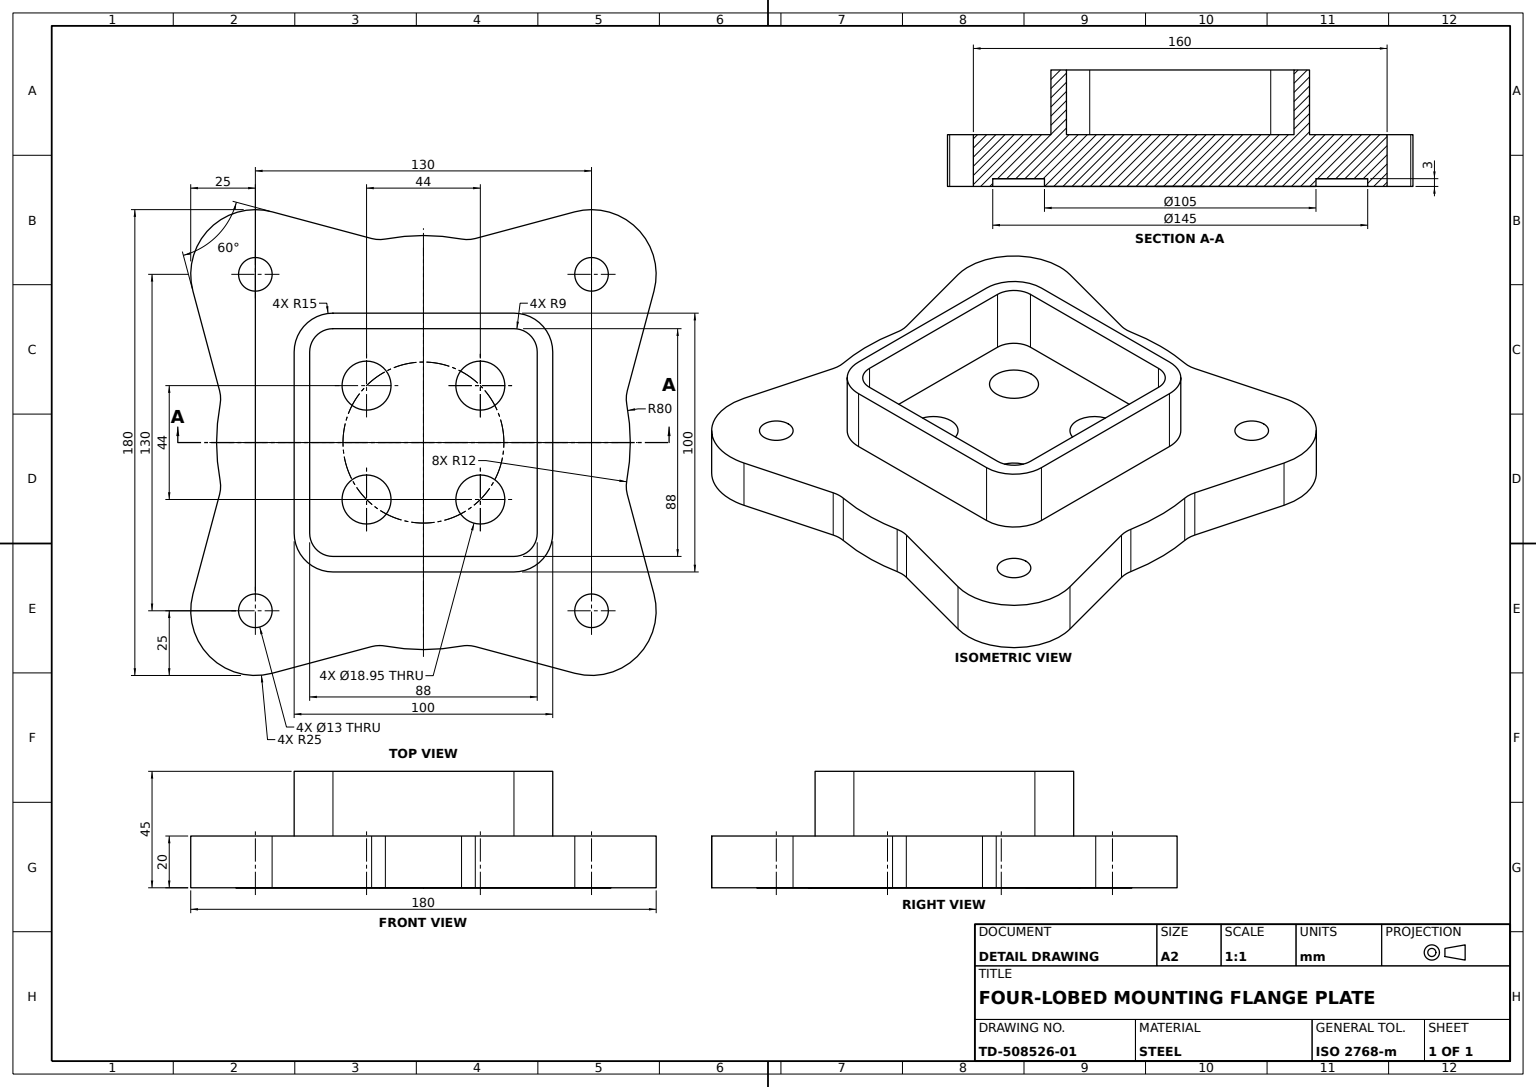
SolidWorks part; units mm, degrees
material "Plain Carbon Steel"
ref_plane "Front Plane" through (0, 0, 0) normal (0, 0, 1) x (1, 0, 0)
ref_plane "Top Plane" through (0, 0, 0) normal (0, 1, 0) x (1, 0, 0)
ref_plane "Right Plane" through (0, 0, 0) normal (1, 0, 0) x (0, 0, -1)
sketch "Base Flange Sketch" plane through (0, 0, 0) normal (0, 1, 0) x (1, 0, 0)
  line L0 (-187.1656, 0) -> (144.2241, 0) construction
  line L1 (0, 135.6121) -> (0, -142.8618) construction
  line L2 (0, 0) -> (95.3316, 95.3316) construction
  line L3 (0, 0) -> (95.3316, -95.3316) construction
  line L4 (0, 0) -> (-95.3316, -95.3316) construction
  line L5 (0, 0) -> (-95.3316, 95.3316) construction
  line L6 (-89.1481, 58.5295) -> (-78.8361, 20.0445)
  line L7 (-58.5295, 89.1481) -> (-20.0445, 78.8361)
  line L8 (58.5295, 89.1481) -> (20.0445, 78.8361)
  line L9 (89.1481, 58.5295) -> (78.8361, 20.0445)
  line L10 (89.1481, -58.5295) -> (78.8361, -20.0445)
  line L11 (58.5295, -89.1481) -> (20.0445, -78.8361)
  line L12 (-58.5295, -89.1481) -> (-20.0445, -78.8361)
  line L13 (-89.1481, -58.5295) -> (-78.8361, -20.0445)
  arc A0 (-78.6324, 14.7293) -> (-78.6324, -14.7293) centre (0, 0) ccw
  arc A1 (-58.5295, 89.1481) -> (-89.1481, 58.5295) centre (-65, 65) ccw
  arc A2 (89.1481, 58.5295) -> (58.5295, 89.1481) centre (65, 65) ccw
  arc A3 (58.5295, -89.1481) -> (89.1481, -58.5295) centre (65, -65) ccw
  arc A4 (-89.1481, -58.5295) -> (-58.5295, -89.1481) centre (-65, -65) ccw
  arc A5 (14.7293, 78.6324) -> (-14.7293, 78.6324) centre (0, 0) ccw
  arc A6 (78.6324, -14.7293) -> (78.6324, 14.7293) centre (0, 0) ccw
  arc A7 (-14.7293, -78.6324) -> (14.7293, -78.6324) centre (0, 0) ccw
  arc A8 (20.0445, -78.8361) -> (14.7293, -78.6324) centre (16.9387, -90.4272) ccw
  arc A9 (-20.0445, -78.8361) -> (-14.7293, -78.6324) centre (-16.9387, -90.4272) cw
  arc A10 (-78.8361, -20.0445) -> (-78.6324, -14.7293) centre (-90.4272, -16.9387) ccw
  arc A11 (78.8361, -20.0445) -> (78.6324, -14.7293) centre (90.4272, -16.9387) cw
  arc A12 (78.8361, 20.0445) -> (78.6324, 14.7293) centre (90.4272, 16.9387) ccw
  arc A13 (-78.6324, 14.7293) -> (-78.8361, 20.0445) centre (-90.4272, 16.9387) ccw
  arc A14 (20.0445, 78.8361) -> (14.7293, 78.6324) centre (16.9387, 90.4272) cw
  arc A15 (-14.7293, 78.6324) -> (-20.0445, 78.8361) centre (-16.9387, 90.4272) cw
  circle A16 centre (-65, 65) radius 6.5
  circle A17 centre (65, 65) radius 6.5
  circle A18 centre (65, -65) radius 6.5
  circle A19 centre (-65, -65) radius 6.5
  point P22 (0, 0)
  point P37 (0, 0)
  point P58 (0, 0)
  dimension "D1" = 160
  dimension "D2" = 50
  dimension "D16" = 12
  dimension "D18" = 13
  dimension "D3" = 65
  dimension "D4" = 65
  dimension "D5" = 65
  dimension "D6" = 65
  dimension "D7" = 65
  dimension "D8" = 65
  dimension "D9" = 65
  dimension "D10" = 65
  dimension "D12" = 60
  dimension "D13" = 30
  dimension "D14" = 30
  dimension "D15" = 75
  dimension "D19" = 187.1656
  dimension "D20" = 144.2241
  dimension "D21" = 135.6121
  dimension "D22" = 142.8618
  dimension "D11" = 4
  dimension "D17" = 4
extrude "Base Flange" add sketch "Base Flange Sketch" along normal mid plane 20
sketch "Square Boss Sketch" plane through (0, 10, 0) normal (0, 1, 0) x (1, 0, 0)
  line L1 (-35, 50) -> (35, 50)
  line L2 (-50, 35) -> (-50, -35)
  line L3 (-35, -50) -> (35, -50)
  line L4 (50, 35) -> (50, -35)
  line L5 (-50, 50) -> (50, -50) construction
  line L6 (-50, -50) -> (50, 50) construction
  line L10 (-44, 35) -> (-44, -35)
  line L11 (-35, -44) -> (35, -44)
  line L12 (44, 35) -> (44, -35)
  line L13 (-35, 44) -> (35, 44)
  circle A0 centre (-22, 22) radius 9.4731
  circle A1 centre (22, 22) radius 9.4731
  circle A2 centre (22, -22) radius 9.4731
  circle A3 centre (-22, -22) radius 9.4731
  arc A4 (-50, -35) -> (-35, -50) centre (-35, -35) ccw
  arc A5 (35, -50) -> (50, -35) centre (35, -35) ccw
  arc A6 (35, 50) -> (50, 35) centre (35, 35) cw
  arc A7 (-35, 50) -> (-50, 35) centre (-35, 35) ccw
  arc A8 (-44, -35) -> (-35, -44) centre (-35, -35) ccw
  arc A9 (35, -44) -> (44, -35) centre (35, -35) ccw
  arc A10 (35, 44) -> (44, 35) centre (35, 35) cw
  arc A11 (-35, 44) -> (-44, 35) centre (-35, 35) ccw
  point P0 (0, 0)
  dimension "D3" = 15
  dimension "D13" = 18.9462
  dimension "D1" = 100
  dimension "D2" = 100
  dimension "D4" = 44
  dimension "D5" = 44
  dimension "D6" = 22
  dimension "D7" = 22
  dimension "D8" = 22
  dimension "D9" = 44
  dimension "D10" = 44
  dimension "D11" = 22
  dimension "D12" = 6
extrude "Square Boss" add sketch "Square Boss Sketch" along normal blind 25 contours L1 A7 L2 A4 L3 A5 L4 A6 A11 L13 A10 L12 A9 L11 A8 L10
sketch "Boss Pocket Sketch" plane through (0, 10, 0) normal (0, 1, 0) x (1, 0, 0)
  circle A0 centre (-22, -22) radius 9.4731 construction
  circle A1 centre (22, -22) radius 9.4731 construction
  circle A2 centre (22, 22) radius 9.4731 construction
  circle A3 centre (-22, 22) radius 9.4731 construction
  circle A4 centre (-22, -22) radius 9.4731
  circle A5 centre (22, -22) radius 9.4731
  circle A6 centre (22, 22) radius 9.4731
  circle A7 centre (-22, 22) radius 9.4731
extrude "Boss Pocket" cut sketch "Boss Pocket Sketch" against normal through all both and the other way through all
sketch "Recess Sketch" plane through (0, -10, 0) normal (0, -1, 0) x (1, 0, 0)
  circle A0 centre (0, 0) radius 52.5
  circle A1 centre (0, 0) radius 72.5
  dimension "D1" = 105
  dimension "D2" = 145
extrude "Recess Cut 3mm" cut sketch "Recess Sketch" against normal blind 3 and the other way through all
